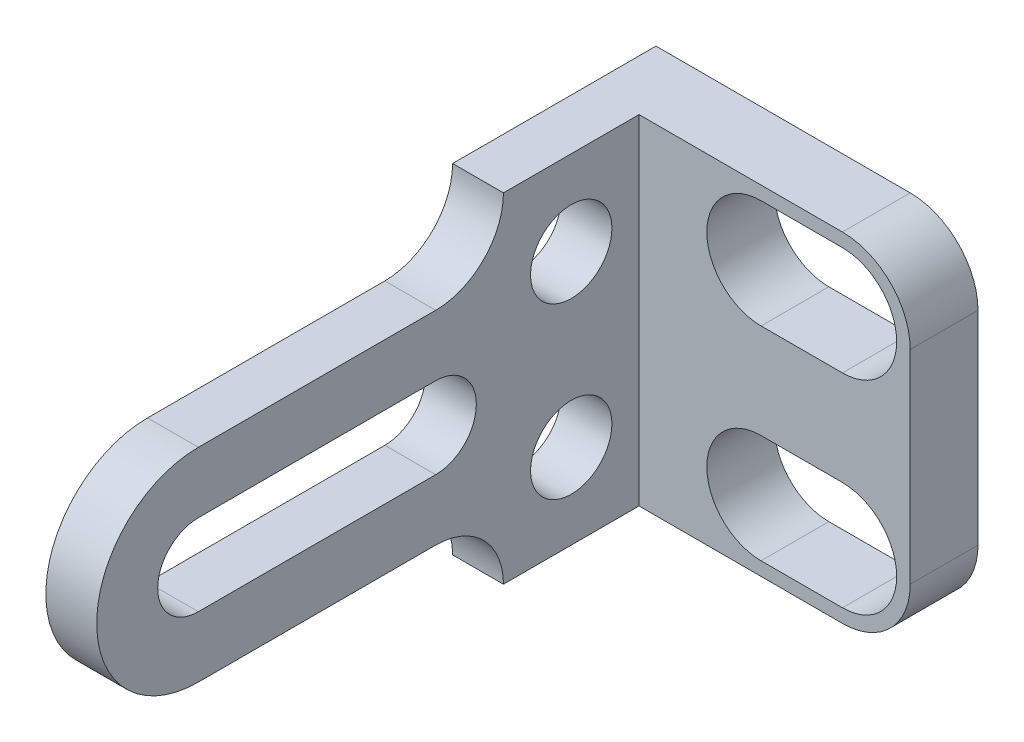
ISO-10303-21;
HEADER;
FILE_DESCRIPTION(('STEP AP214'),'2;1');
FILE_NAME('part.step','',(''),(''),'','','');
FILE_SCHEMA(('AUTOMOTIVE_DESIGN { 1 0 10303 214 1 1 1 1 }'));
ENDSEC;
DATA;
#1=APPLICATION_CONTEXT('core data for automotive mechanical design processes');
#2=APPLICATION_PROTOCOL_DEFINITION('international standard','automotive_design',2000,#1);
#3=PRODUCT_CONTEXT('',#1,'mechanical');
#4=PRODUCT('Part','Part','',(#3));
#5=PRODUCT_RELATED_PRODUCT_CATEGORY('part','',(#4));
#6=PRODUCT_DEFINITION_FORMATION('','',#4);
#7=PRODUCT_DEFINITION_CONTEXT('part definition',#1,'design');
#8=PRODUCT_DEFINITION('design','',#6,#7);
#9=PRODUCT_DEFINITION_SHAPE('','',#8);
#10=(LENGTH_UNIT() NAMED_UNIT(*) SI_UNIT(.MILLI.,.METRE.));
#11=(NAMED_UNIT(*) PLANE_ANGLE_UNIT() SI_UNIT($,.RADIAN.));
#12=(NAMED_UNIT(*) SI_UNIT($,.STERADIAN.) SOLID_ANGLE_UNIT());
#13=UNCERTAINTY_MEASURE_WITH_UNIT(LENGTH_MEASURE(1.E-05),#10,'distance_accuracy_value','');
#14=(GEOMETRIC_REPRESENTATION_CONTEXT(3) GLOBAL_UNCERTAINTY_ASSIGNED_CONTEXT((#13)) GLOBAL_UNIT_ASSIGNED_CONTEXT((#10,
#11,#12)) REPRESENTATION_CONTEXT('',''));
#15=CARTESIAN_POINT('',(0.,0.,0.));
#16=DIRECTION('',(0.,0.,1.));
#17=DIRECTION('',(1.,0.,0.));
#18=AXIS2_PLACEMENT_3D('',#15,#16,#17);
#19=CARTESIAN_POINT('',(0.,0.,20.));
#20=DIRECTION('',(0.,1.,0.));
#21=DIRECTION('',(0.,0.,1.));
#22=AXIS2_PLACEMENT_3D('',#19,#20,#21);
#23=PLANE('',#22);
#24=DIRECTION('',(1.,0.,0.));
#25=VECTOR('',#24,1.);
#26=CARTESIAN_POINT('',(0.,0.,0.));
#27=LINE('',#26,#25);
#28=CARTESIAN_POINT('',(-15.,0.,0.));
#29=VERTEX_POINT('',#28);
#30=CARTESIAN_POINT('',(59.9999999999999,0.,0.));
#31=VERTEX_POINT('',#30);
#32=EDGE_CURVE('E374',#29,#31,#27,.T.);
#33=ORIENTED_EDGE('',*,*,#32,.T.);
#34=DIRECTION('',(0.,0.,-1.));
#35=VECTOR('',#34,1.);
#36=CARTESIAN_POINT('',(59.9999999999999,0.,20.));
#37=LINE('',#36,#35);
#38=CARTESIAN_POINT('',(59.9999999999999,0.,20.));
#39=VERTEX_POINT('',#38);
#40=EDGE_CURVE('E11',#39,#31,#37,.T.);
#41=ORIENTED_EDGE('',*,*,#40,.F.);
#42=DIRECTION('',(1.,0.,0.));
#43=VECTOR('',#42,1.);
#44=CARTESIAN_POINT('',(0.,0.,20.));
#45=LINE('',#44,#43);
#46=CARTESIAN_POINT('',(0.,0.,20.));
#47=VERTEX_POINT('',#46);
#48=EDGE_CURVE('E377',#47,#39,#45,.T.);
#49=ORIENTED_EDGE('',*,*,#48,.F.);
#50=DIRECTION('',(0.,0.,1.));
#51=VECTOR('',#50,1.);
#52=CARTESIAN_POINT('',(0.,0.,20.));
#53=LINE('',#52,#51);
#54=CARTESIAN_POINT('',(0.,0.,60.));
#55=VERTEX_POINT('',#54);
#56=EDGE_CURVE('E352',#47,#55,#53,.T.);
#57=ORIENTED_EDGE('',*,*,#56,.T.);
#58=DIRECTION('',(1.,0.,0.));
#59=VECTOR('',#58,1.);
#60=CARTESIAN_POINT('',(-15.,0.,60.));
#61=LINE('',#60,#59);
#62=CARTESIAN_POINT('',(-15.,0.,60.));
#63=VERTEX_POINT('',#62);
#64=EDGE_CURVE('E375',#63,#55,#61,.T.);
#65=ORIENTED_EDGE('',*,*,#64,.F.);
#66=DIRECTION('',(0.,0.,1.));
#67=VECTOR('',#66,1.);
#68=CARTESIAN_POINT('',(-15.,0.,0.));
#69=LINE('',#68,#67);
#70=EDGE_CURVE('E360',#29,#63,#69,.T.);
#71=ORIENTED_EDGE('',*,*,#70,.F.);
#72=EDGE_LOOP('',(#33,#41,#49,#57,#65,#71));
#73=FACE_BOUND('',#72,.T.);
#74=ADVANCED_FACE('F44',(#73),#23,.F.);
#75=CARTESIAN_POINT('',(60.,20.,20.));
#76=DIRECTION('',(0.,0.,-1.));
#77=DIRECTION('',(-1.,0.,0.));
#78=AXIS2_PLACEMENT_3D('',#75,#76,#77);
#79=CYLINDRICAL_SURFACE('',#78,20.);
#80=CARTESIAN_POINT('',(60.,20.,0.));
#81=DIRECTION('',(0.,0.,1.));
#82=DIRECTION('',(1.,0.,0.));
#83=AXIS2_PLACEMENT_3D('',#80,#81,#82);
#84=CIRCLE('',#83,20.);
#85=CARTESIAN_POINT('',(80.,20.,0.));
#86=VERTEX_POINT('',#85);
#87=EDGE_CURVE('E393',#31,#86,#84,.T.);
#88=ORIENTED_EDGE('',*,*,#87,.T.);
#89=DIRECTION('',(0.,0.,-1.));
#90=VECTOR('',#89,1.);
#91=CARTESIAN_POINT('',(80.,20.,20.));
#92=LINE('',#91,#90);
#93=CARTESIAN_POINT('',(80.,20.,20.));
#94=VERTEX_POINT('',#93);
#95=EDGE_CURVE('E55',#94,#86,#92,.T.);
#96=ORIENTED_EDGE('',*,*,#95,.F.);
#97=CARTESIAN_POINT('',(60.,20.,20.));
#98=DIRECTION('',(0.,0.,1.));
#99=DIRECTION('',(1.,0.,0.));
#100=AXIS2_PLACEMENT_3D('',#97,#98,#99);
#101=CIRCLE('',#100,20.);
#102=EDGE_CURVE('E385',#39,#94,#101,.T.);
#103=ORIENTED_EDGE('',*,*,#102,.F.);
#104=ORIENTED_EDGE('',*,*,#40,.T.);
#105=EDGE_LOOP('',(#88,#96,#103,#104));
#106=FACE_BOUND('',#105,.T.);
#107=ADVANCED_FACE('F427',(#106),#79,.T.);
#108=CARTESIAN_POINT('',(80.,20.0000000000001,20.));
#109=DIRECTION('',(-1.,0.,0.));
#110=DIRECTION('',(0.,0.,1.));
#111=AXIS2_PLACEMENT_3D('',#108,#109,#110);
#112=PLANE('',#111);
#113=DIRECTION('',(0.,1.,0.));
#114=VECTOR('',#113,1.);
#115=CARTESIAN_POINT('',(80.,20.0000000000001,0.));
#116=LINE('',#115,#114);
#117=CARTESIAN_POINT('',(80.,79.9999999999999,0.));
#118=VERTEX_POINT('',#117);
#119=EDGE_CURVE('E391',#86,#118,#116,.T.);
#120=ORIENTED_EDGE('',*,*,#119,.T.);
#121=DIRECTION('',(0.,0.,-1.));
#122=VECTOR('',#121,1.);
#123=CARTESIAN_POINT('',(80.,79.9999999999999,20.));
#124=LINE('',#123,#122);
#125=CARTESIAN_POINT('',(80.,79.9999999999999,20.));
#126=VERTEX_POINT('',#125);
#127=EDGE_CURVE('E405',#126,#118,#124,.T.);
#128=ORIENTED_EDGE('',*,*,#127,.F.);
#129=DIRECTION('',(0.,1.,0.));
#130=VECTOR('',#129,1.);
#131=CARTESIAN_POINT('',(80.,20.0000000000001,20.));
#132=LINE('',#131,#130);
#133=EDGE_CURVE('E383',#94,#126,#132,.T.);
#134=ORIENTED_EDGE('',*,*,#133,.F.);
#135=ORIENTED_EDGE('',*,*,#95,.T.);
#136=EDGE_LOOP('',(#120,#128,#134,#135));
#137=FACE_BOUND('',#136,.T.);
#138=ADVANCED_FACE('F409',(#137),#112,.F.);
#139=CARTESIAN_POINT('',(60.,80.,20.));
#140=DIRECTION('',(0.,0.,-1.));
#141=DIRECTION('',(-1.,0.,0.));
#142=AXIS2_PLACEMENT_3D('',#139,#140,#141);
#143=CYLINDRICAL_SURFACE('',#142,20.);
#144=CARTESIAN_POINT('',(60.,80.,0.));
#145=DIRECTION('',(0.,0.,1.));
#146=DIRECTION('',(-1.,0.,0.));
#147=AXIS2_PLACEMENT_3D('',#144,#145,#146);
#148=CIRCLE('',#147,20.);
#149=CARTESIAN_POINT('',(59.9999999999999,100.,0.));
#150=VERTEX_POINT('',#149);
#151=EDGE_CURVE('E400',#118,#150,#148,.T.);
#152=ORIENTED_EDGE('',*,*,#151,.T.);
#153=DIRECTION('',(0.,0.,-1.));
#154=VECTOR('',#153,1.);
#155=CARTESIAN_POINT('',(59.9999999999999,100.,20.));
#156=LINE('',#155,#154);
#157=CARTESIAN_POINT('',(59.9999999999999,100.,20.));
#158=VERTEX_POINT('',#157);
#159=EDGE_CURVE('E392',#158,#150,#156,.T.);
#160=ORIENTED_EDGE('',*,*,#159,.F.);
#161=CARTESIAN_POINT('',(60.,80.,20.));
#162=DIRECTION('',(0.,0.,1.));
#163=DIRECTION('',(-1.,0.,0.));
#164=AXIS2_PLACEMENT_3D('',#161,#162,#163);
#165=CIRCLE('',#164,20.);
#166=EDGE_CURVE('E387',#126,#158,#165,.T.);
#167=ORIENTED_EDGE('',*,*,#166,.F.);
#168=ORIENTED_EDGE('',*,*,#127,.T.);
#169=EDGE_LOOP('',(#152,#160,#167,#168));
#170=FACE_BOUND('',#169,.T.);
#171=ADVANCED_FACE('F419',(#170),#143,.T.);
#172=CARTESIAN_POINT('',(59.9999999999999,100.,20.));
#173=DIRECTION('',(0.,-1.,0.));
#174=DIRECTION('',(0.,0.,-1.));
#175=AXIS2_PLACEMENT_3D('',#172,#173,#174);
#176=PLANE('',#175);
#177=DIRECTION('',(-1.,0.,0.));
#178=VECTOR('',#177,1.);
#179=CARTESIAN_POINT('',(59.9999999999999,100.,0.));
#180=LINE('',#179,#178);
#181=CARTESIAN_POINT('',(-15.,100.,0.));
#182=VERTEX_POINT('',#181);
#183=EDGE_CURVE('E379',#150,#182,#180,.T.);
#184=ORIENTED_EDGE('',*,*,#183,.T.);
#185=DIRECTION('',(0.,0.,-1.));
#186=VECTOR('',#185,1.);
#187=CARTESIAN_POINT('',(-15.,100.,60.));
#188=LINE('',#187,#186);
#189=CARTESIAN_POINT('',(-15.,100.,60.));
#190=VERTEX_POINT('',#189);
#191=EDGE_CURVE('E357',#190,#182,#188,.T.);
#192=ORIENTED_EDGE('',*,*,#191,.F.);
#193=DIRECTION('',(1.,0.,0.));
#194=VECTOR('',#193,1.);
#195=CARTESIAN_POINT('',(-15.,100.,60.));
#196=LINE('',#195,#194);
#197=CARTESIAN_POINT('',(0.,100.,60.));
#198=VERTEX_POINT('',#197);
#199=EDGE_CURVE('E368',#190,#198,#196,.T.);
#200=ORIENTED_EDGE('',*,*,#199,.T.);
#201=DIRECTION('',(0.,0.,-1.));
#202=VECTOR('',#201,1.);
#203=CARTESIAN_POINT('',(0.,100.,60.));
#204=LINE('',#203,#202);
#205=CARTESIAN_POINT('',(0.,100.,20.));
#206=VERTEX_POINT('',#205);
#207=EDGE_CURVE('E359',#198,#206,#204,.T.);
#208=ORIENTED_EDGE('',*,*,#207,.T.);
#209=DIRECTION('',(-1.,0.,0.));
#210=VECTOR('',#209,1.);
#211=CARTESIAN_POINT('',(59.9999999999999,100.,20.));
#212=LINE('',#211,#210);
#213=EDGE_CURVE('E389',#158,#206,#212,.T.);
#214=ORIENTED_EDGE('',*,*,#213,.F.);
#215=ORIENTED_EDGE('',*,*,#159,.T.);
#216=EDGE_LOOP('',(#184,#192,#200,#208,#214,#215));
#217=FACE_BOUND('',#216,.T.);
#218=ADVANCED_FACE('F424',(#217),#176,.F.);
#219=CARTESIAN_POINT('',(60.,20.,20.));
#220=DIRECTION('',(0.,0.,1.));
#221=DIRECTION('',(1.,0.,0.));
#222=AXIS2_PLACEMENT_3D('',#219,#220,#221);
#223=PLANE('',#222);
#224=CARTESIAN_POINT('',(36.,80.,20.));
#225=DIRECTION('',(0.,0.,1.));
#226=DIRECTION('',(1.,0.,0.));
#227=AXIS2_PLACEMENT_3D('',#224,#225,#226);
#228=CIRCLE('',#227,16.);
#229=CARTESIAN_POINT('',(36.,96.,20.));
#230=VERTEX_POINT('',#229);
#231=CARTESIAN_POINT('',(36.,64.,20.));
#232=VERTEX_POINT('',#231);
#233=EDGE_CURVE('E56',#230,#232,#228,.T.);
#234=ORIENTED_EDGE('',*,*,#233,.F.);
#235=DIRECTION('',(-1.,0.,0.));
#236=VECTOR('',#235,1.);
#237=CARTESIAN_POINT('',(36.,96.,20.));
#238=LINE('',#237,#236);
#239=CARTESIAN_POINT('',(60.,96.,20.));
#240=VERTEX_POINT('',#239);
#241=EDGE_CURVE('E227',#240,#230,#238,.T.);
#242=ORIENTED_EDGE('',*,*,#241,.F.);
#243=CARTESIAN_POINT('',(60.,80.,20.));
#244=DIRECTION('',(0.,0.,1.));
#245=DIRECTION('',(1.,0.,0.));
#246=AXIS2_PLACEMENT_3D('',#243,#244,#245);
#247=CIRCLE('',#246,16.);
#248=CARTESIAN_POINT('',(60.,64.,20.));
#249=VERTEX_POINT('',#248);
#250=EDGE_CURVE('E229',#249,#240,#247,.T.);
#251=ORIENTED_EDGE('',*,*,#250,.F.);
#252=DIRECTION('',(1.,0.,0.));
#253=VECTOR('',#252,1.);
#254=CARTESIAN_POINT('',(60.,64.,20.));
#255=LINE('',#254,#253);
#256=EDGE_CURVE('E234',#232,#249,#255,.T.);
#257=ORIENTED_EDGE('',*,*,#256,.F.);
#258=EDGE_LOOP('',(#234,#242,#251,#257));
#259=FACE_BOUND('',#258,.T.);
#260=CARTESIAN_POINT('',(36.,20.,20.));
#261=DIRECTION('',(0.,0.,1.));
#262=DIRECTION('',(1.,0.,0.));
#263=AXIS2_PLACEMENT_3D('',#260,#261,#262);
#264=CIRCLE('',#263,16.);
#265=CARTESIAN_POINT('',(36.,36.,20.));
#266=VERTEX_POINT('',#265);
#267=CARTESIAN_POINT('',(36.,3.99999999999999,20.));
#268=VERTEX_POINT('',#267);
#269=EDGE_CURVE('E70',#266,#268,#264,.T.);
#270=ORIENTED_EDGE('',*,*,#269,.F.);
#271=DIRECTION('',(-1.,0.,0.));
#272=VECTOR('',#271,1.);
#273=CARTESIAN_POINT('',(36.,36.,20.));
#274=LINE('',#273,#272);
#275=CARTESIAN_POINT('',(60.,36.,20.));
#276=VERTEX_POINT('',#275);
#277=EDGE_CURVE('E249',#276,#266,#274,.T.);
#278=ORIENTED_EDGE('',*,*,#277,.F.);
#279=CARTESIAN_POINT('',(60.,20.,20.));
#280=DIRECTION('',(0.,0.,1.));
#281=DIRECTION('',(1.,0.,0.));
#282=AXIS2_PLACEMENT_3D('',#279,#280,#281);
#283=CIRCLE('',#282,16.);
#284=CARTESIAN_POINT('',(60.,3.99999999999999,20.));
#285=VERTEX_POINT('',#284);
#286=EDGE_CURVE('E262',#285,#276,#283,.T.);
#287=ORIENTED_EDGE('',*,*,#286,.F.);
#288=DIRECTION('',(1.,0.,0.));
#289=VECTOR('',#288,1.);
#290=CARTESIAN_POINT('',(60.,3.99999999999999,20.));
#291=LINE('',#290,#289);
#292=EDGE_CURVE('E261',#268,#285,#291,.T.);
#293=ORIENTED_EDGE('',*,*,#292,.F.);
#294=EDGE_LOOP('',(#270,#278,#287,#293));
#295=FACE_BOUND('',#294,.T.);
#296=DIRECTION('',(0.,-1.,0.));
#297=VECTOR('',#296,1.);
#298=CARTESIAN_POINT('',(0.,100.,20.));
#299=LINE('',#298,#297);
#300=EDGE_CURVE('E376',#206,#47,#299,.T.);
#301=ORIENTED_EDGE('',*,*,#300,.T.);
#302=ORIENTED_EDGE('',*,*,#48,.T.);
#303=ORIENTED_EDGE('',*,*,#102,.T.);
#304=ORIENTED_EDGE('',*,*,#133,.T.);
#305=ORIENTED_EDGE('',*,*,#166,.T.);
#306=ORIENTED_EDGE('',*,*,#213,.T.);
#307=EDGE_LOOP('',(#301,#302,#303,#304,#305,#306));
#308=FACE_BOUND('',#307,.T.);
#309=ADVANCED_FACE('F426',(#259,#295,#308),#223,.T.);
#310=CARTESIAN_POINT('',(60.,20.,0.));
#311=DIRECTION('',(0.,0.,1.));
#312=DIRECTION('',(1.,0.,0.));
#313=AXIS2_PLACEMENT_3D('',#310,#311,#312);
#314=PLANE('',#313);
#315=DIRECTION('',(-1.,0.,0.));
#316=VECTOR('',#315,1.);
#317=CARTESIAN_POINT('',(36.,96.,0.));
#318=LINE('',#317,#316);
#319=CARTESIAN_POINT('',(60.,96.,0.));
#320=VERTEX_POINT('',#319);
#321=CARTESIAN_POINT('',(36.,96.,0.));
#322=VERTEX_POINT('',#321);
#323=EDGE_CURVE('E213',#320,#322,#318,.T.);
#324=ORIENTED_EDGE('',*,*,#323,.T.);
#325=CARTESIAN_POINT('',(36.,80.,0.));
#326=DIRECTION('',(0.,0.,1.));
#327=DIRECTION('',(1.,0.,0.));
#328=AXIS2_PLACEMENT_3D('',#325,#326,#327);
#329=CIRCLE('',#328,16.);
#330=CARTESIAN_POINT('',(36.,64.,0.));
#331=VERTEX_POINT('',#330);
#332=EDGE_CURVE('E210',#322,#331,#329,.T.);
#333=ORIENTED_EDGE('',*,*,#332,.T.);
#334=DIRECTION('',(1.,0.,0.));
#335=VECTOR('',#334,1.);
#336=CARTESIAN_POINT('',(60.,64.,0.));
#337=LINE('',#336,#335);
#338=CARTESIAN_POINT('',(60.,64.,0.));
#339=VERTEX_POINT('',#338);
#340=EDGE_CURVE('E220',#331,#339,#337,.T.);
#341=ORIENTED_EDGE('',*,*,#340,.T.);
#342=CARTESIAN_POINT('',(60.,80.,0.));
#343=DIRECTION('',(0.,0.,1.));
#344=DIRECTION('',(1.,0.,0.));
#345=AXIS2_PLACEMENT_3D('',#342,#343,#344);
#346=CIRCLE('',#345,16.);
#347=EDGE_CURVE('E222',#339,#320,#346,.T.);
#348=ORIENTED_EDGE('',*,*,#347,.T.);
#349=EDGE_LOOP('',(#324,#333,#341,#348));
#350=FACE_BOUND('',#349,.T.);
#351=DIRECTION('',(-1.,0.,0.));
#352=VECTOR('',#351,1.);
#353=CARTESIAN_POINT('',(36.,36.,0.));
#354=LINE('',#353,#352);
#355=CARTESIAN_POINT('',(60.,36.,0.));
#356=VERTEX_POINT('',#355);
#357=CARTESIAN_POINT('',(36.,36.,0.));
#358=VERTEX_POINT('',#357);
#359=EDGE_CURVE('E258',#356,#358,#354,.T.);
#360=ORIENTED_EDGE('',*,*,#359,.T.);
#361=CARTESIAN_POINT('',(36.,20.,0.));
#362=DIRECTION('',(0.,0.,1.));
#363=DIRECTION('',(1.,0.,0.));
#364=AXIS2_PLACEMENT_3D('',#361,#362,#363);
#365=CIRCLE('',#364,16.);
#366=CARTESIAN_POINT('',(36.,3.99999999999999,0.));
#367=VERTEX_POINT('',#366);
#368=EDGE_CURVE('E248',#358,#367,#365,.T.);
#369=ORIENTED_EDGE('',*,*,#368,.T.);
#370=DIRECTION('',(1.,0.,0.));
#371=VECTOR('',#370,1.);
#372=CARTESIAN_POINT('',(60.,3.99999999999999,0.));
#373=LINE('',#372,#371);
#374=CARTESIAN_POINT('',(60.,3.99999999999999,0.));
#375=VERTEX_POINT('',#374);
#376=EDGE_CURVE('E247',#367,#375,#373,.T.);
#377=ORIENTED_EDGE('',*,*,#376,.T.);
#378=CARTESIAN_POINT('',(60.,20.,0.));
#379=DIRECTION('',(0.,0.,1.));
#380=DIRECTION('',(1.,0.,0.));
#381=AXIS2_PLACEMENT_3D('',#378,#379,#380);
#382=CIRCLE('',#381,16.);
#383=EDGE_CURVE('E251',#375,#356,#382,.T.);
#384=ORIENTED_EDGE('',*,*,#383,.T.);
#385=EDGE_LOOP('',(#360,#369,#377,#384));
#386=FACE_BOUND('',#385,.T.);
#387=ORIENTED_EDGE('',*,*,#32,.F.);
#388=DIRECTION('',(0.,-1.,0.));
#389=VECTOR('',#388,1.);
#390=CARTESIAN_POINT('',(-15.,100.,0.));
#391=LINE('',#390,#389);
#392=EDGE_CURVE('E361',#182,#29,#391,.T.);
#393=ORIENTED_EDGE('',*,*,#392,.F.);
#394=ORIENTED_EDGE('',*,*,#183,.F.);
#395=ORIENTED_EDGE('',*,*,#151,.F.);
#396=ORIENTED_EDGE('',*,*,#119,.F.);
#397=ORIENTED_EDGE('',*,*,#87,.F.);
#398=EDGE_LOOP('',(#387,#393,#394,#395,#396,#397));
#399=FACE_BOUND('',#398,.T.);
#400=ADVANCED_FACE('F224',(#350,#386,#399),#314,.F.);
#401=CARTESIAN_POINT('',(-15.,0.,0.));
#402=DIRECTION('',(-1.,0.,0.));
#403=DIRECTION('',(0.,0.,1.));
#404=AXIS2_PLACEMENT_3D('',#401,#402,#403);
#405=PLANE('',#404);
#406=CARTESIAN_POINT('',(-15.,75.,40.));
#407=DIRECTION('',(1.,0.,0.));
#408=DIRECTION('',(0.,0.,-1.));
#409=AXIS2_PLACEMENT_3D('',#406,#407,#408);
#410=CIRCLE('',#409,12.);
#411=CARTESIAN_POINT('',(-15.,75.,28.));
#412=VERTEX_POINT('',#411);
#413=EDGE_CURVE('E274',#412,#412,#410,.T.);
#414=ORIENTED_EDGE('',*,*,#413,.T.);
#415=EDGE_LOOP('',(#414));
#416=FACE_BOUND('',#415,.T.);
#417=CARTESIAN_POINT('',(-15.,25.,40.));
#418=DIRECTION('',(1.,0.,0.));
#419=DIRECTION('',(0.,0.,-1.));
#420=AXIS2_PLACEMENT_3D('',#417,#418,#419);
#421=CIRCLE('',#420,12.);
#422=CARTESIAN_POINT('',(-15.,25.,28.));
#423=VERTEX_POINT('',#422);
#424=EDGE_CURVE('E285',#423,#423,#421,.T.);
#425=ORIENTED_EDGE('',*,*,#424,.T.);
#426=EDGE_LOOP('',(#425));
#427=FACE_BOUND('',#426,.T.);
#428=ORIENTED_EDGE('',*,*,#70,.T.);
#429=CARTESIAN_POINT('',(-15.,0.,80.));
#430=DIRECTION('',(1.,0.,0.));
#431=DIRECTION('',(0.,0.,1.));
#432=AXIS2_PLACEMENT_3D('',#429,#430,#431);
#433=CIRCLE('',#432,20.);
#434=CARTESIAN_POINT('',(-15.,20.,80.));
#435=VERTEX_POINT('',#434);
#436=EDGE_CURVE('E342',#63,#435,#433,.T.);
#437=ORIENTED_EDGE('',*,*,#436,.T.);
#438=DIRECTION('',(0.,0.,1.));
#439=VECTOR('',#438,1.);
#440=CARTESIAN_POINT('',(-15.,20.,150.));
#441=LINE('',#440,#439);
#442=CARTESIAN_POINT('',(-15.,20.,150.));
#443=VERTEX_POINT('',#442);
#444=EDGE_CURVE('E323',#435,#443,#441,.T.);
#445=ORIENTED_EDGE('',*,*,#444,.T.);
#446=CARTESIAN_POINT('',(-15.,50.,150.));
#447=DIRECTION('',(-1.,0.,0.));
#448=DIRECTION('',(0.,0.,1.));
#449=AXIS2_PLACEMENT_3D('',#446,#447,#448);
#450=CIRCLE('',#449,30.);
#451=CARTESIAN_POINT('',(-15.,80.,150.));
#452=VERTEX_POINT('',#451);
#453=EDGE_CURVE('E315',#443,#452,#450,.T.);
#454=ORIENTED_EDGE('',*,*,#453,.T.);
#455=DIRECTION('',(0.,0.,-1.));
#456=VECTOR('',#455,1.);
#457=CARTESIAN_POINT('',(-15.,80.,150.));
#458=LINE('',#457,#456);
#459=CARTESIAN_POINT('',(-15.,80.,80.));
#460=VERTEX_POINT('',#459);
#461=EDGE_CURVE('E338',#452,#460,#458,.T.);
#462=ORIENTED_EDGE('',*,*,#461,.T.);
#463=CARTESIAN_POINT('',(-15.,100.,80.));
#464=DIRECTION('',(1.,0.,0.));
#465=DIRECTION('',(0.,0.,-1.));
#466=AXIS2_PLACEMENT_3D('',#463,#464,#465);
#467=CIRCLE('',#466,20.);
#468=EDGE_CURVE('E343',#460,#190,#467,.T.);
#469=ORIENTED_EDGE('',*,*,#468,.T.);
#470=ORIENTED_EDGE('',*,*,#191,.T.);
#471=ORIENTED_EDGE('',*,*,#392,.T.);
#472=EDGE_LOOP('',(#428,#437,#445,#454,#462,#469,#470,#471));
#473=FACE_BOUND('',#472,.T.);
#474=CARTESIAN_POINT('',(-15.,50.,80.));
#475=DIRECTION('',(-1.,0.,0.));
#476=DIRECTION('',(0.,0.,1.));
#477=AXIS2_PLACEMENT_3D('',#474,#475,#476);
#478=CIRCLE('',#477,12.);
#479=CARTESIAN_POINT('',(-15.,62.,80.));
#480=VERTEX_POINT('',#479);
#481=CARTESIAN_POINT('',(-15.,38.,80.));
#482=VERTEX_POINT('',#481);
#483=EDGE_CURVE('E279',#480,#482,#478,.T.);
#484=ORIENTED_EDGE('',*,*,#483,.F.);
#485=DIRECTION('',(0.,0.,-1.));
#486=VECTOR('',#485,1.);
#487=CARTESIAN_POINT('',(-15.,62.,80.));
#488=LINE('',#487,#486);
#489=CARTESIAN_POINT('',(-15.,62.,150.));
#490=VERTEX_POINT('',#489);
#491=EDGE_CURVE('E292',#490,#480,#488,.T.);
#492=ORIENTED_EDGE('',*,*,#491,.F.);
#493=CARTESIAN_POINT('',(-15.,50.,150.));
#494=DIRECTION('',(-1.,0.,0.));
#495=DIRECTION('',(0.,0.,1.));
#496=AXIS2_PLACEMENT_3D('',#493,#494,#495);
#497=CIRCLE('',#496,12.);
#498=CARTESIAN_POINT('',(-15.,38.,150.));
#499=VERTEX_POINT('',#498);
#500=EDGE_CURVE('E304',#499,#490,#497,.T.);
#501=ORIENTED_EDGE('',*,*,#500,.F.);
#502=DIRECTION('',(0.,0.,1.));
#503=VECTOR('',#502,1.);
#504=CARTESIAN_POINT('',(-15.,38.,150.));
#505=LINE('',#504,#503);
#506=EDGE_CURVE('E305',#482,#499,#505,.T.);
#507=ORIENTED_EDGE('',*,*,#506,.F.);
#508=EDGE_LOOP('',(#484,#492,#501,#507));
#509=FACE_BOUND('',#508,.T.);
#510=ADVANCED_FACE('F432',(#416,#427,#473,#509),#405,.T.);
#511=CARTESIAN_POINT('',(0.,0.,0.));
#512=DIRECTION('',(-1.,0.,0.));
#513=DIRECTION('',(0.,0.,1.));
#514=AXIS2_PLACEMENT_3D('',#511,#512,#513);
#515=PLANE('',#514);
#516=CARTESIAN_POINT('',(0.,75.,40.));
#517=DIRECTION('',(1.,0.,0.));
#518=DIRECTION('',(0.,0.,-1.));
#519=AXIS2_PLACEMENT_3D('',#516,#517,#518);
#520=CIRCLE('',#519,12.);
#521=CARTESIAN_POINT('',(0.,75.,28.));
#522=VERTEX_POINT('',#521);
#523=EDGE_CURVE('E276',#522,#522,#520,.T.);
#524=ORIENTED_EDGE('',*,*,#523,.F.);
#525=EDGE_LOOP('',(#524));
#526=FACE_BOUND('',#525,.T.);
#527=CARTESIAN_POINT('',(0.,25.,40.));
#528=DIRECTION('',(1.,0.,0.));
#529=DIRECTION('',(0.,0.,-1.));
#530=AXIS2_PLACEMENT_3D('',#527,#528,#529);
#531=CIRCLE('',#530,12.);
#532=CARTESIAN_POINT('',(0.,25.,28.));
#533=VERTEX_POINT('',#532);
#534=EDGE_CURVE('E245',#533,#533,#531,.T.);
#535=ORIENTED_EDGE('',*,*,#534,.F.);
#536=EDGE_LOOP('',(#535));
#537=FACE_BOUND('',#536,.T.);
#538=ORIENTED_EDGE('',*,*,#300,.F.);
#539=ORIENTED_EDGE('',*,*,#207,.F.);
#540=CARTESIAN_POINT('',(0.,100.,80.));
#541=DIRECTION('',(1.,0.,0.));
#542=DIRECTION('',(0.,0.,-1.));
#543=AXIS2_PLACEMENT_3D('',#540,#541,#542);
#544=CIRCLE('',#543,20.);
#545=CARTESIAN_POINT('',(0.,80.,80.));
#546=VERTEX_POINT('',#545);
#547=EDGE_CURVE('E326',#546,#198,#544,.T.);
#548=ORIENTED_EDGE('',*,*,#547,.F.);
#549=DIRECTION('',(0.,0.,-1.));
#550=VECTOR('',#549,1.);
#551=CARTESIAN_POINT('',(0.,80.,150.));
#552=LINE('',#551,#550);
#553=CARTESIAN_POINT('',(0.,80.,150.));
#554=VERTEX_POINT('',#553);
#555=EDGE_CURVE('E325',#554,#546,#552,.T.);
#556=ORIENTED_EDGE('',*,*,#555,.F.);
#557=CARTESIAN_POINT('',(0.,50.,150.));
#558=DIRECTION('',(-1.,0.,0.));
#559=DIRECTION('',(0.,0.,1.));
#560=AXIS2_PLACEMENT_3D('',#557,#558,#559);
#561=CIRCLE('',#560,30.);
#562=CARTESIAN_POINT('',(0.,20.,150.));
#563=VERTEX_POINT('',#562);
#564=EDGE_CURVE('E317',#563,#554,#561,.T.);
#565=ORIENTED_EDGE('',*,*,#564,.F.);
#566=DIRECTION('',(0.,0.,1.));
#567=VECTOR('',#566,1.);
#568=CARTESIAN_POINT('',(0.,20.,150.));
#569=LINE('',#568,#567);
#570=CARTESIAN_POINT('',(0.,20.,80.));
#571=VERTEX_POINT('',#570);
#572=EDGE_CURVE('E335',#571,#563,#569,.T.);
#573=ORIENTED_EDGE('',*,*,#572,.F.);
#574=CARTESIAN_POINT('',(0.,0.,80.));
#575=DIRECTION('',(1.,0.,0.));
#576=DIRECTION('',(0.,0.,1.));
#577=AXIS2_PLACEMENT_3D('',#574,#575,#576);
#578=CIRCLE('',#577,20.);
#579=EDGE_CURVE('E328',#55,#571,#578,.T.);
#580=ORIENTED_EDGE('',*,*,#579,.F.);
#581=ORIENTED_EDGE('',*,*,#56,.F.);
#582=EDGE_LOOP('',(#538,#539,#548,#556,#565,#573,#580,#581));
#583=FACE_BOUND('',#582,.T.);
#584=DIRECTION('',(0.,0.,-1.));
#585=VECTOR('',#584,1.);
#586=CARTESIAN_POINT('',(0.,62.,80.));
#587=LINE('',#586,#585);
#588=CARTESIAN_POINT('',(0.,62.,150.));
#589=VERTEX_POINT('',#588);
#590=CARTESIAN_POINT('',(0.,62.,80.));
#591=VERTEX_POINT('',#590);
#592=EDGE_CURVE('E300',#589,#591,#587,.T.);
#593=ORIENTED_EDGE('',*,*,#592,.T.);
#594=CARTESIAN_POINT('',(0.,50.,80.));
#595=DIRECTION('',(-1.,0.,0.));
#596=DIRECTION('',(0.,0.,1.));
#597=AXIS2_PLACEMENT_3D('',#594,#595,#596);
#598=CIRCLE('',#597,12.);
#599=CARTESIAN_POINT('',(0.,38.,80.));
#600=VERTEX_POINT('',#599);
#601=EDGE_CURVE('E290',#591,#600,#598,.T.);
#602=ORIENTED_EDGE('',*,*,#601,.T.);
#603=DIRECTION('',(0.,0.,1.));
#604=VECTOR('',#603,1.);
#605=CARTESIAN_POINT('',(0.,38.,150.));
#606=LINE('',#605,#604);
#607=CARTESIAN_POINT('',(0.,38.,150.));
#608=VERTEX_POINT('',#607);
#609=EDGE_CURVE('E289',#600,#608,#606,.T.);
#610=ORIENTED_EDGE('',*,*,#609,.T.);
#611=CARTESIAN_POINT('',(0.,50.,150.));
#612=DIRECTION('',(-1.,0.,0.));
#613=DIRECTION('',(0.,0.,1.));
#614=AXIS2_PLACEMENT_3D('',#611,#612,#613);
#615=CIRCLE('',#614,12.);
#616=EDGE_CURVE('E294',#608,#589,#615,.T.);
#617=ORIENTED_EDGE('',*,*,#616,.T.);
#618=EDGE_LOOP('',(#593,#602,#610,#617));
#619=FACE_BOUND('',#618,.T.);
#620=ADVANCED_FACE('F444',(#526,#537,#583,#619),#515,.F.);
#621=CARTESIAN_POINT('',(0.,50.,150.));
#622=DIRECTION('',(-1.,0.,0.));
#623=DIRECTION('',(0.,0.,1.));
#624=AXIS2_PLACEMENT_3D('',#621,#622,#623);
#625=CYLINDRICAL_SURFACE('',#624,30.);
#626=ORIENTED_EDGE('',*,*,#453,.F.);
#627=DIRECTION('',(-1.,0.,0.));
#628=VECTOR('',#627,1.);
#629=CARTESIAN_POINT('',(0.,20.,150.));
#630=LINE('',#629,#628);
#631=EDGE_CURVE('E349',#563,#443,#630,.T.);
#632=ORIENTED_EDGE('',*,*,#631,.F.);
#633=ORIENTED_EDGE('',*,*,#564,.T.);
#634=DIRECTION('',(-1.,0.,0.));
#635=VECTOR('',#634,1.);
#636=CARTESIAN_POINT('',(0.,80.,150.));
#637=LINE('',#636,#635);
#638=EDGE_CURVE('E333',#554,#452,#637,.T.);
#639=ORIENTED_EDGE('',*,*,#638,.T.);
#640=EDGE_LOOP('',(#626,#632,#633,#639));
#641=FACE_BOUND('',#640,.T.);
#642=ADVANCED_FACE('F453',(#641),#625,.T.);
#643=CARTESIAN_POINT('',(0.,20.,150.));
#644=DIRECTION('',(0.,-1.,0.));
#645=DIRECTION('',(0.,0.,-1.));
#646=AXIS2_PLACEMENT_3D('',#643,#644,#645);
#647=PLANE('',#646);
#648=ORIENTED_EDGE('',*,*,#444,.F.);
#649=DIRECTION('',(-1.,0.,0.));
#650=VECTOR('',#649,1.);
#651=CARTESIAN_POINT('',(0.,20.,80.));
#652=LINE('',#651,#650);
#653=EDGE_CURVE('E355',#571,#435,#652,.T.);
#654=ORIENTED_EDGE('',*,*,#653,.F.);
#655=ORIENTED_EDGE('',*,*,#572,.T.);
#656=ORIENTED_EDGE('',*,*,#631,.T.);
#657=EDGE_LOOP('',(#648,#654,#655,#656));
#658=FACE_BOUND('',#657,.T.);
#659=ADVANCED_FACE('F457',(#658),#647,.T.);
#660=CARTESIAN_POINT('',(0.,0.,80.));
#661=DIRECTION('',(-1.,0.,0.));
#662=DIRECTION('',(0.,0.,1.));
#663=AXIS2_PLACEMENT_3D('',#660,#661,#662);
#664=CYLINDRICAL_SURFACE('',#663,20.);
#665=ORIENTED_EDGE('',*,*,#436,.F.);
#666=ORIENTED_EDGE('',*,*,#64,.T.);
#667=ORIENTED_EDGE('',*,*,#579,.T.);
#668=ORIENTED_EDGE('',*,*,#653,.T.);
#669=EDGE_LOOP('',(#665,#666,#667,#668));
#670=FACE_BOUND('',#669,.T.);
#671=ADVANCED_FACE('F459',(#670),#664,.F.);
#672=CARTESIAN_POINT('',(0.,100.,80.));
#673=DIRECTION('',(-1.,0.,0.));
#674=DIRECTION('',(0.,0.,1.));
#675=AXIS2_PLACEMENT_3D('',#672,#673,#674);
#676=CYLINDRICAL_SURFACE('',#675,20.);
#677=ORIENTED_EDGE('',*,*,#468,.F.);
#678=DIRECTION('',(-1.,0.,0.));
#679=VECTOR('',#678,1.);
#680=CARTESIAN_POINT('',(0.,80.,80.));
#681=LINE('',#680,#679);
#682=EDGE_CURVE('E354',#546,#460,#681,.T.);
#683=ORIENTED_EDGE('',*,*,#682,.F.);
#684=ORIENTED_EDGE('',*,*,#547,.T.);
#685=ORIENTED_EDGE('',*,*,#199,.F.);
#686=EDGE_LOOP('',(#677,#683,#684,#685));
#687=FACE_BOUND('',#686,.T.);
#688=ADVANCED_FACE('F438',(#687),#676,.F.);
#689=CARTESIAN_POINT('',(0.,80.,150.));
#690=DIRECTION('',(0.,1.,0.));
#691=DIRECTION('',(0.,0.,1.));
#692=AXIS2_PLACEMENT_3D('',#689,#690,#691);
#693=PLANE('',#692);
#694=ORIENTED_EDGE('',*,*,#461,.F.);
#695=ORIENTED_EDGE('',*,*,#638,.F.);
#696=ORIENTED_EDGE('',*,*,#555,.T.);
#697=ORIENTED_EDGE('',*,*,#682,.T.);
#698=EDGE_LOOP('',(#694,#695,#696,#697));
#699=FACE_BOUND('',#698,.T.);
#700=ADVANCED_FACE('F448',(#699),#693,.T.);
#701=CARTESIAN_POINT('',(0.,50.,80.));
#702=DIRECTION('',(-1.,0.,0.));
#703=DIRECTION('',(0.,0.,1.));
#704=AXIS2_PLACEMENT_3D('',#701,#702,#703);
#705=CYLINDRICAL_SURFACE('',#704,12.);
#706=ORIENTED_EDGE('',*,*,#483,.T.);
#707=DIRECTION('',(-1.,0.,0.));
#708=VECTOR('',#707,1.);
#709=CARTESIAN_POINT('',(0.,38.,80.));
#710=LINE('',#709,#708);
#711=EDGE_CURVE('E296',#600,#482,#710,.T.);
#712=ORIENTED_EDGE('',*,*,#711,.F.);
#713=ORIENTED_EDGE('',*,*,#601,.F.);
#714=DIRECTION('',(-1.,0.,0.));
#715=VECTOR('',#714,1.);
#716=CARTESIAN_POINT('',(0.,62.,80.));
#717=LINE('',#716,#715);
#718=EDGE_CURVE('E309',#591,#480,#717,.T.);
#719=ORIENTED_EDGE('',*,*,#718,.T.);
#720=EDGE_LOOP('',(#706,#712,#713,#719));
#721=FACE_BOUND('',#720,.T.);
#722=ADVANCED_FACE('F494',(#721),#705,.F.);
#723=CARTESIAN_POINT('',(0.,62.,80.));
#724=DIRECTION('',(0.,1.,0.));
#725=DIRECTION('',(0.,0.,1.));
#726=AXIS2_PLACEMENT_3D('',#723,#724,#725);
#727=PLANE('',#726);
#728=ORIENTED_EDGE('',*,*,#491,.T.);
#729=ORIENTED_EDGE('',*,*,#718,.F.);
#730=ORIENTED_EDGE('',*,*,#592,.F.);
#731=DIRECTION('',(-1.,0.,0.));
#732=VECTOR('',#731,1.);
#733=CARTESIAN_POINT('',(0.,62.,150.));
#734=LINE('',#733,#732);
#735=EDGE_CURVE('E311',#589,#490,#734,.T.);
#736=ORIENTED_EDGE('',*,*,#735,.T.);
#737=EDGE_LOOP('',(#728,#729,#730,#736));
#738=FACE_BOUND('',#737,.T.);
#739=ADVANCED_FACE('F496',(#738),#727,.F.);
#740=CARTESIAN_POINT('',(0.,50.,150.));
#741=DIRECTION('',(-1.,0.,0.));
#742=DIRECTION('',(0.,0.,1.));
#743=AXIS2_PLACEMENT_3D('',#740,#741,#742);
#744=CYLINDRICAL_SURFACE('',#743,12.);
#745=ORIENTED_EDGE('',*,*,#500,.T.);
#746=ORIENTED_EDGE('',*,*,#735,.F.);
#747=ORIENTED_EDGE('',*,*,#616,.F.);
#748=DIRECTION('',(-1.,0.,0.));
#749=VECTOR('',#748,1.);
#750=CARTESIAN_POINT('',(0.,38.,150.));
#751=LINE('',#750,#749);
#752=EDGE_CURVE('E312',#608,#499,#751,.T.);
#753=ORIENTED_EDGE('',*,*,#752,.T.);
#754=EDGE_LOOP('',(#745,#746,#747,#753));
#755=FACE_BOUND('',#754,.T.);
#756=ADVANCED_FACE('F501',(#755),#744,.F.);
#757=CARTESIAN_POINT('',(0.,38.,150.));
#758=DIRECTION('',(0.,-1.,0.));
#759=DIRECTION('',(0.,0.,-1.));
#760=AXIS2_PLACEMENT_3D('',#757,#758,#759);
#761=PLANE('',#760);
#762=ORIENTED_EDGE('',*,*,#506,.T.);
#763=ORIENTED_EDGE('',*,*,#752,.F.);
#764=ORIENTED_EDGE('',*,*,#609,.F.);
#765=ORIENTED_EDGE('',*,*,#711,.T.);
#766=EDGE_LOOP('',(#762,#763,#764,#765));
#767=FACE_BOUND('',#766,.T.);
#768=ADVANCED_FACE('F507',(#767),#761,.F.);
#769=CARTESIAN_POINT('',(-15.,25.,40.));
#770=DIRECTION('',(1.,0.,0.));
#771=DIRECTION('',(0.,0.,-1.));
#772=AXIS2_PLACEMENT_3D('',#769,#770,#771);
#773=CYLINDRICAL_SURFACE('',#772,12.);
#774=ORIENTED_EDGE('',*,*,#424,.F.);
#775=EDGE_LOOP('',(#774));
#776=FACE_BOUND('',#775,.T.);
#777=ORIENTED_EDGE('',*,*,#534,.T.);
#778=EDGE_LOOP('',(#777));
#779=FACE_BOUND('',#778,.T.);
#780=ADVANCED_FACE('F515',(#776,#779),#773,.F.);
#781=CARTESIAN_POINT('',(-15.,75.,40.));
#782=DIRECTION('',(1.,0.,0.));
#783=DIRECTION('',(0.,0.,-1.));
#784=AXIS2_PLACEMENT_3D('',#781,#782,#783);
#785=CYLINDRICAL_SURFACE('',#784,12.);
#786=ORIENTED_EDGE('',*,*,#413,.F.);
#787=EDGE_LOOP('',(#786));
#788=FACE_BOUND('',#787,.T.);
#789=ORIENTED_EDGE('',*,*,#523,.T.);
#790=EDGE_LOOP('',(#789));
#791=FACE_BOUND('',#790,.T.);
#792=ADVANCED_FACE('F519',(#788,#791),#785,.F.);
#793=CARTESIAN_POINT('',(36.,20.,0.));
#794=DIRECTION('',(0.,0.,1.));
#795=DIRECTION('',(1.,0.,0.));
#796=AXIS2_PLACEMENT_3D('',#793,#794,#795);
#797=CYLINDRICAL_SURFACE('',#796,16.);
#798=ORIENTED_EDGE('',*,*,#269,.T.);
#799=DIRECTION('',(0.,0.,1.));
#800=VECTOR('',#799,1.);
#801=CARTESIAN_POINT('',(36.,3.99999999999999,0.));
#802=LINE('',#801,#800);
#803=EDGE_CURVE('E259',#367,#268,#802,.T.);
#804=ORIENTED_EDGE('',*,*,#803,.F.);
#805=ORIENTED_EDGE('',*,*,#368,.F.);
#806=DIRECTION('',(0.,0.,1.));
#807=VECTOR('',#806,1.);
#808=CARTESIAN_POINT('',(36.,36.,0.));
#809=LINE('',#808,#807);
#810=EDGE_CURVE('E237',#358,#266,#809,.T.);
#811=ORIENTED_EDGE('',*,*,#810,.T.);
#812=EDGE_LOOP('',(#798,#804,#805,#811));
#813=FACE_BOUND('',#812,.T.);
#814=ADVANCED_FACE('F521',(#813),#797,.F.);
#815=CARTESIAN_POINT('',(36.,36.,0.));
#816=DIRECTION('',(0.,1.,0.));
#817=DIRECTION('',(0.,0.,1.));
#818=AXIS2_PLACEMENT_3D('',#815,#816,#817);
#819=PLANE('',#818);
#820=ORIENTED_EDGE('',*,*,#277,.T.);
#821=ORIENTED_EDGE('',*,*,#810,.F.);
#822=ORIENTED_EDGE('',*,*,#359,.F.);
#823=DIRECTION('',(0.,0.,1.));
#824=VECTOR('',#823,1.);
#825=CARTESIAN_POINT('',(60.,36.,0.));
#826=LINE('',#825,#824);
#827=EDGE_CURVE('E269',#356,#276,#826,.T.);
#828=ORIENTED_EDGE('',*,*,#827,.T.);
#829=EDGE_LOOP('',(#820,#821,#822,#828));
#830=FACE_BOUND('',#829,.T.);
#831=ADVANCED_FACE('F527',(#830),#819,.F.);
#832=CARTESIAN_POINT('',(60.,20.,0.));
#833=DIRECTION('',(0.,0.,1.));
#834=DIRECTION('',(1.,0.,0.));
#835=AXIS2_PLACEMENT_3D('',#832,#833,#834);
#836=CYLINDRICAL_SURFACE('',#835,16.);
#837=ORIENTED_EDGE('',*,*,#286,.T.);
#838=ORIENTED_EDGE('',*,*,#827,.F.);
#839=ORIENTED_EDGE('',*,*,#383,.F.);
#840=DIRECTION('',(0.,0.,1.));
#841=VECTOR('',#840,1.);
#842=CARTESIAN_POINT('',(60.,3.99999999999999,0.));
#843=LINE('',#842,#841);
#844=EDGE_CURVE('E275',#375,#285,#843,.T.);
#845=ORIENTED_EDGE('',*,*,#844,.T.);
#846=EDGE_LOOP('',(#837,#838,#839,#845));
#847=FACE_BOUND('',#846,.T.);
#848=ADVANCED_FACE('F533',(#847),#836,.F.);
#849=CARTESIAN_POINT('',(60.,3.99999999999999,0.));
#850=DIRECTION('',(0.,-1.,0.));
#851=DIRECTION('',(0.,0.,-1.));
#852=AXIS2_PLACEMENT_3D('',#849,#850,#851);
#853=PLANE('',#852);
#854=ORIENTED_EDGE('',*,*,#292,.T.);
#855=ORIENTED_EDGE('',*,*,#844,.F.);
#856=ORIENTED_EDGE('',*,*,#376,.F.);
#857=ORIENTED_EDGE('',*,*,#803,.T.);
#858=EDGE_LOOP('',(#854,#855,#856,#857));
#859=FACE_BOUND('',#858,.T.);
#860=ADVANCED_FACE('F526',(#859),#853,.F.);
#861=CARTESIAN_POINT('',(36.,80.,0.));
#862=DIRECTION('',(0.,0.,1.));
#863=DIRECTION('',(1.,0.,0.));
#864=AXIS2_PLACEMENT_3D('',#861,#862,#863);
#865=CYLINDRICAL_SURFACE('',#864,16.);
#866=ORIENTED_EDGE('',*,*,#233,.T.);
#867=DIRECTION('',(0.,0.,1.));
#868=VECTOR('',#867,1.);
#869=CARTESIAN_POINT('',(36.,64.,0.));
#870=LINE('',#869,#868);
#871=EDGE_CURVE('E201',#331,#232,#870,.T.);
#872=ORIENTED_EDGE('',*,*,#871,.F.);
#873=ORIENTED_EDGE('',*,*,#332,.F.);
#874=DIRECTION('',(0.,0.,1.));
#875=VECTOR('',#874,1.);
#876=CARTESIAN_POINT('',(36.,96.,0.));
#877=LINE('',#876,#875);
#878=EDGE_CURVE('E238',#322,#230,#877,.T.);
#879=ORIENTED_EDGE('',*,*,#878,.T.);
#880=EDGE_LOOP('',(#866,#872,#873,#879));
#881=FACE_BOUND('',#880,.T.);
#882=ADVANCED_FACE('F202',(#881),#865,.F.);
#883=CARTESIAN_POINT('',(36.,96.,0.));
#884=DIRECTION('',(0.,1.,0.));
#885=DIRECTION('',(0.,0.,1.));
#886=AXIS2_PLACEMENT_3D('',#883,#884,#885);
#887=PLANE('',#886);
#888=ORIENTED_EDGE('',*,*,#241,.T.);
#889=ORIENTED_EDGE('',*,*,#878,.F.);
#890=ORIENTED_EDGE('',*,*,#323,.F.);
#891=DIRECTION('',(0.,0.,1.));
#892=VECTOR('',#891,1.);
#893=CARTESIAN_POINT('',(60.,96.,0.));
#894=LINE('',#893,#892);
#895=EDGE_CURVE('E243',#320,#240,#894,.T.);
#896=ORIENTED_EDGE('',*,*,#895,.T.);
#897=EDGE_LOOP('',(#888,#889,#890,#896));
#898=FACE_BOUND('',#897,.T.);
#899=ADVANCED_FACE('F541',(#898),#887,.F.);
#900=CARTESIAN_POINT('',(60.,80.,0.));
#901=DIRECTION('',(0.,0.,1.));
#902=DIRECTION('',(1.,0.,0.));
#903=AXIS2_PLACEMENT_3D('',#900,#901,#902);
#904=CYLINDRICAL_SURFACE('',#903,16.);
#905=ORIENTED_EDGE('',*,*,#250,.T.);
#906=ORIENTED_EDGE('',*,*,#895,.F.);
#907=ORIENTED_EDGE('',*,*,#347,.F.);
#908=DIRECTION('',(0.,0.,1.));
#909=VECTOR('',#908,1.);
#910=CARTESIAN_POINT('',(60.,64.,0.));
#911=LINE('',#910,#909);
#912=EDGE_CURVE('E215',#339,#249,#911,.T.);
#913=ORIENTED_EDGE('',*,*,#912,.T.);
#914=EDGE_LOOP('',(#905,#906,#907,#913));
#915=FACE_BOUND('',#914,.T.);
#916=ADVANCED_FACE('F542',(#915),#904,.F.);
#917=CARTESIAN_POINT('',(60.,64.,0.));
#918=DIRECTION('',(0.,-1.,0.));
#919=DIRECTION('',(0.,0.,-1.));
#920=AXIS2_PLACEMENT_3D('',#917,#918,#919);
#921=PLANE('',#920);
#922=ORIENTED_EDGE('',*,*,#256,.T.);
#923=ORIENTED_EDGE('',*,*,#912,.F.);
#924=ORIENTED_EDGE('',*,*,#340,.F.);
#925=ORIENTED_EDGE('',*,*,#871,.T.);
#926=EDGE_LOOP('',(#922,#923,#924,#925));
#927=FACE_BOUND('',#926,.T.);
#928=ADVANCED_FACE('F217',(#927),#921,.F.);
#929=CLOSED_SHELL('',(#74,#107,#138,#171,#218,#309,#400,#510,#620,#642,#659,#671,#688,#700,#722,
#739,#756,#768,#780,#792,#814,#831,#848,#860,#882,#899,#916,#928));
#930=MANIFOLD_SOLID_BREP('B2',#929);
#931=ADVANCED_BREP_SHAPE_REPRESENTATION('',(#18,#930),#14);
#932=SHAPE_DEFINITION_REPRESENTATION(#9,#931);
ENDSEC;
END-ISO-10303-21;
